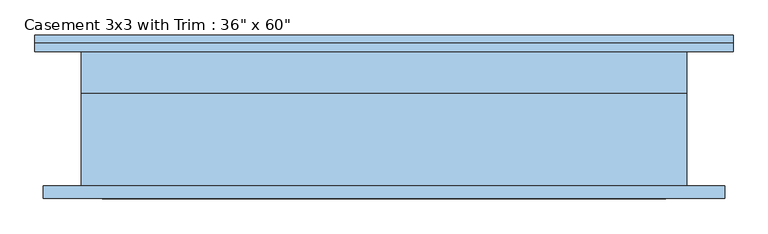
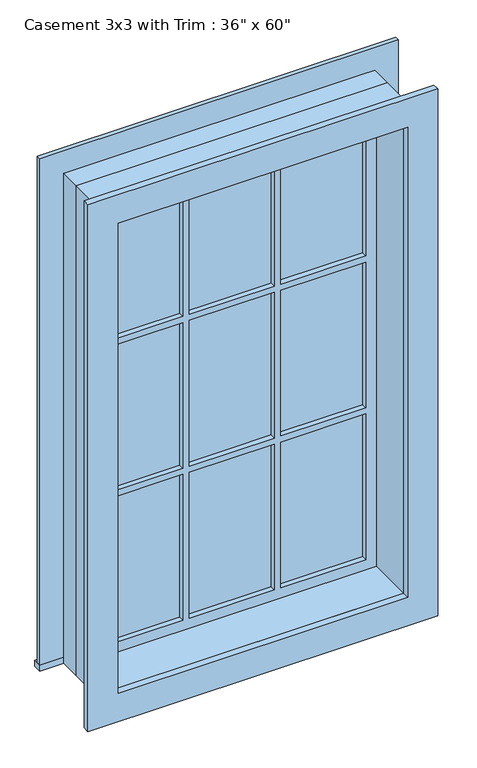
"""IFC4 building model written with IfcOpenShell, lengths in millimetres: window geometry."""

from ifc_helpers import new_model, si_unit, frame, origin, place, context, project, spatial, polyline, outline, extrude, source, transform, mapped, element, save


def window_58e1470a(model_context):
    return source(origin(), model_context, "Body", "SweptSolid", [
        extrude(outline(polyline([(-527.05, 127.0), (527.05, 127.0), (527.05, 101.6), (-527.05, 101.6), (-527.05, 127.0)])), frame((0.0, 0.0, 609.6), z_axis=(0.0, 0.0, 1.0), x_axis=(1.0, 0.0, 0.0)), (0.0, 0.0, 1.0), 19.05),
        extrude(outline(polyline([(2114.55, -438.15), (2114.55, 438.15), (628.65, 438.15), (628.65, 527.05), (2203.45, 527.05), (2203.45, -527.05), (628.65, -527.05), (628.65, -438.15), (2114.55, -438.15)])), frame((0.0, 101.6, 0.0), z_axis=(0.0, 1.0, 0.0), x_axis=(0.0, 0.0, 1.0)), (0.0, 0.0, 1.0), 12.7),
        extrude(outline(polyline([(143.9333333, 66.675), (393.7, 66.675), (393.7, 53.975), (143.9333333, 53.975), (143.9333333, 66.675)])), frame((0.0, 0.0, 1617.1333333), z_axis=(0.0, 0.0, 1.0), x_axis=(1.0, 0.0, 0.0)), (0.0, 0.0, 1.0), 452.9666667),
        extrude(outline(polyline([(-124.8833333, 66.675), (124.8833333, 66.675), (124.8833333, 53.975), (-124.8833333, 53.975), (-124.8833333, 66.675)])), frame((0.0, 0.0, 1617.1333333), z_axis=(0.0, 0.0, 1.0), x_axis=(1.0, 0.0, 0.0)), (0.0, 0.0, 1.0), 452.9666667),
        extrude(outline(polyline([(-393.7, 66.675), (-143.9333333, 66.675), (-143.9333333, 53.975), (-393.7, 53.975), (-393.7, 66.675)])), frame((0.0, 0.0, 1617.1333333), z_axis=(0.0, 0.0, 1.0), x_axis=(1.0, 0.0, 0.0)), (0.0, 0.0, 1.0), 452.9666667),
        extrude(outline(polyline([(-393.7, 66.675), (-143.9333333, 66.675), (-143.9333333, 53.975), (-393.7, 53.975), (-393.7, 66.675)])), frame((0.0, 0.0, 1145.1166667), z_axis=(0.0, 0.0, 1.0), x_axis=(1.0, 0.0, 0.0)), (0.0, 0.0, 1.0), 452.9666667),
        extrude(outline(polyline([(-124.8833333, 66.675), (124.8833333, 66.675), (124.8833333, 53.975), (-124.8833333, 53.975), (-124.8833333, 66.675)])), frame((0.0, 0.0, 1145.1166667), z_axis=(0.0, 0.0, 1.0), x_axis=(1.0, 0.0, 0.0)), (0.0, 0.0, 1.0), 452.9666667),
        extrude(outline(polyline([(143.9333333, 66.675), (393.7, 66.675), (393.7, 53.975), (143.9333333, 53.975), (143.9333333, 66.675)])), frame((0.0, 0.0, 1145.1166667), z_axis=(0.0, 0.0, 1.0), x_axis=(1.0, 0.0, 0.0)), (0.0, 0.0, 1.0), 452.9666667),
        extrude(outline(polyline([(143.9333333, 66.675), (393.7, 66.675), (393.7, 53.975), (143.9333333, 53.975), (143.9333333, 66.675)])), frame((0.0, 0.0, 673.1), z_axis=(0.0, 0.0, 1.0), x_axis=(1.0, 0.0, 0.0)), (0.0, 0.0, 1.0), 452.9666667),
        extrude(outline(polyline([(-124.8833333, 66.675), (124.8833333, 66.675), (124.8833333, 53.975), (-124.8833333, 53.975), (-124.8833333, 66.675)])), frame((0.0, 0.0, 673.1), z_axis=(0.0, 0.0, 1.0), x_axis=(1.0, 0.0, 0.0)), (0.0, 0.0, 1.0), 452.9666667),
        extrude(outline(polyline([(-393.7, 66.675), (-143.9333333, 66.675), (-143.9333333, 53.975), (-393.7, 53.975), (-393.7, 66.675)])), frame((0.0, 0.0, 673.1), z_axis=(0.0, 0.0, 1.0), x_axis=(1.0, 0.0, 0.0)), (0.0, 0.0, 1.0), 452.9666667),
        extrude(outline(polyline([(2190.75, 514.35), (2190.75, -514.35), (552.45, -514.35), (552.45, 514.35), (2190.75, 514.35)]), holes=[polyline([(2101.85, 425.45), (641.35, 425.45), (641.35, -425.45), (2101.85, -425.45), (2101.85, 425.45)])]), frame((0.0, -120.65, 0.0), z_axis=(0.0, 1.0, 0.0), x_axis=(0.0, 0.0, 1.0)), (0.0, 0.0, 1.0), 19.05),
        extrude(outline(polyline([(2114.55, -438.15), (628.65, -438.15), (628.65, 438.15), (2114.55, 438.15), (2114.55, -438.15)]), holes=[polyline([(2070.1, -143.9333333), (1617.1333333, -143.9333333), (1617.1333333, -393.7), (2070.1, -393.7), (2070.1, -143.9333333)]), polyline([(1598.0833333, -143.9333333), (1145.1166667, -143.9333333), (1145.1166667, -393.7), (1598.0833333, -393.7), (1598.0833333, -143.9333333)]), polyline([(1126.0666667, -143.9333333), (673.1, -143.9333333), (673.1, -393.7), (1126.0666667, -393.7), (1126.0666667, -143.9333333)]), polyline([(2070.1, 124.8833333), (1617.1333333, 124.8833333), (1617.1333333, -124.8833333), (2070.1, -124.8833333), (2070.1, 124.8833333)]), polyline([(1598.0833333, 124.8833333), (1145.1166667, 124.8833333), (1145.1166667, -124.8833333), (1598.0833333, -124.8833333), (1598.0833333, 124.8833333)]), polyline([(1126.0666667, 124.8833333), (673.1, 124.8833333), (673.1, -124.8833333), (1126.0666667, -124.8833333), (1126.0666667, 124.8833333)]), polyline([(2070.1, 393.7), (1617.1333333, 393.7), (1617.1333333, 143.9333333), (2070.1, 143.9333333), (2070.1, 393.7)]), polyline([(1598.0833333, 393.7), (1145.1166667, 393.7), (1145.1166667, 143.9333333), (1598.0833333, 143.9333333), (1598.0833333, 393.7)]), polyline([(1126.0666667, 393.7), (673.1, 393.7), (673.1, 143.9333333), (1126.0666667, 143.9333333), (1126.0666667, 393.7)])]), frame((0.0, 38.1, 0.0), z_axis=(0.0, 1.0, 0.0), x_axis=(0.0, 0.0, 1.0)), (0.0, 0.0, 1.0), 44.45),
        extrude(outline(polyline([(2133.6, -457.2), (609.6, -457.2), (609.6, 457.2), (2133.6, 457.2), (2133.6, -457.2)]), holes=[polyline([(2101.85, -425.45), (2101.85, 425.45), (641.35, 425.45), (641.35, -425.45), (2101.85, -425.45)])]), frame((0.0, -101.6, 0.0), z_axis=(0.0, 1.0, 0.0), x_axis=(0.0, 0.0, 1.0)), (0.0, 0.0, 1.0), 139.7),
        extrude(outline(polyline([(2133.6, 457.2), (2133.6, -457.2), (609.6, -457.2), (609.6, 457.2), (2133.6, 457.2)]), holes=[polyline([(2114.55, 438.15), (628.65, 438.15), (628.65, -438.15), (2114.55, -438.15), (2114.55, 438.15)])]), frame((0.0, 38.1, 0.0), z_axis=(0.0, 1.0, 0.0), x_axis=(0.0, 0.0, 1.0)), (0.0, 0.0, 1.0), 63.5),
    ])


if __name__ == "__main__":
    model = new_model("IFC4")
    model_context = context("Model", 3, world=origin())
    ifc_project = project(units=[si_unit("LENGTHUNIT", "METRE", prefix="MILLI")], contexts=[model_context])
    site = spatial("IfcSite", under=ifc_project)
    building = spatial("IfcBuilding", under=site)
    placement = place(None, origin())
    window_shape = window_58e1470a(model_context)
    element("IfcWindow", 1, ObjectType="Casement 3x3 with Trim : 36\" x 60\"", at=placement, inside=building, context=model_context, shape_type="MappedRepresentation", body=[
        mapped(window_shape, transform((0.0, 0.0, 0.0), x_axis=(1.0, 0.0, 0.0), y_axis=(0.0, 1.0, 0.0), z_axis=(0.0, 0.0, 1.0))),
    ])
    save(model, "model.ifc")

# Revit data of these elements
# Type "Casement 3x3 with Trim : 36\" x 60\""
#   Type Mark = "11"
#   Construction Type Id = "GSP4R"
#   Assembly Code = "B2020100"
#   Analytic Construction = "1/8 in Pilkington single glazing"
#   Visual Light Transmittance = 0.9
#   Solar Heat Gain Coefficient = 0.78
#   Heat Transfer Coefficient (U) = 0.6496 BTU/(h·ft²·°F)
#   Height = 5' - 0"
#   Default Sill Height = 2' - 0"
#   Trim Projection - Ext. = 0' - 0 1/2"
#   Trim Projection - Int. = 0' - 0 3/4"
#   Trim Width - Exterior = 0' - 3 1/2"
#   Trim Width - Interior = 0' - 3 1/2"
#   Width = 3' - 0"
#   Window Inset = 0' - 0 3/4"
#   Define Thermal Properties by = 1
#   Glass Pane Material = Glass
#   Sash Material = Sash
#   Trim Exterior Material = Trim
#   Trim Interior Material = Trim
#   Wall Closure = (empty or 0)
# Element 1 (IfcWindow, "Casement 3x3 with Trim : 36\" x 60\"")
#   Materials on its faces: "Sash", "Glass", "Trim"
# Materials
#   "Glass": class "Glass", colour RGB 0 128 192, transparency 0.75, Description = "Soda Lime Glass", Cost = 0
#   "Sash": class "Wood", colour RGB 224 178 126, transparency 0
#   "Trim": class "Wood", colour RGB 224 178 126, transparency 0
